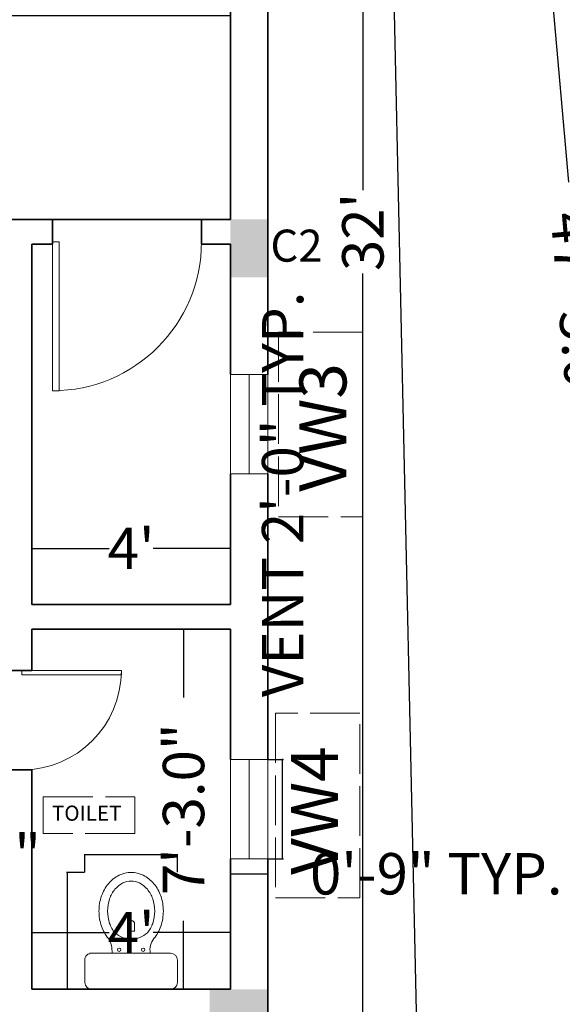
# Model space of a CAD drawing. Units: inches. Extents: x -269 to 4574, y -694 to 313.
# Tile 8 of 19: x 391 to 522, y -360 to -122. Entities that reach past the tile are written whole.
import ezdxf

# ---------------------------------------------------------------- set-up
doc = ezdxf.new("R2010")
doc.units = ezdxf.units.IN
doc.header["$MEASUREMENT"] = 0
doc.linetypes.add('ACAD_ISO02W100', pattern=[15, 12, -3])
for name, color, linetype, lineweight in [('A-ANNO-FRAM', 7, 'ACAD_ISO02W100', 13), ('A-ANNO-IDEN', 6, 'Continuous', 18), ('A-AREA-IDEN', 6, 'Continuous', 20), ('A-COLS', 5, 'Continuous', 35), ('A-COLS-IDEN', 6, 'Continuous', 18), ('A-FLOR-FIXT', 21, 'Continuous', 18), ('C-PROP', 7, 'Continuous', 25), ('DIMENSION', 5, 'Continuous', 18), ('DOORS', 3, 'Continuous', 18), ('WALL', 1, 'Continuous', 35), ('WINDOWS', 2, 'Continuous', 18)]:
    doc.layers.add(name, color=color, linetype=linetype, lineweight=lineweight)
doc.dimstyles.get("Standard").update_dxf_attribs({"dimtxt": 10, "dimasz": 0.18, "dimexe": 0.18, "dimexo": 0.0625, "dimgap": 0.09, "dimtad": 0, "dimdec": 1, "dimzin": 0, "dimdsep": 46, "dimlunit": 3, "dimtxsty": 'Standard', "dimcen": 0.09, "dimclrt": 7, "dimadec": 0, "dimazin": 0, "dimtfac": 1, "dimtdec": 1, "dimtofl": 0, "dimtmove": 0, "dimatfit": 3, "dimfxl": 1, "dimtolj": 1, "dimtzin": 0, "dimarcsym": 0})

# ---------------------------------------------------------------- blocks, each defined once
blk = doc.blocks.new('A$C00A665A6')
for p, q in [((0, 640), (0, 510)), ((40, 680), (500, 680)), ((540, 640), (540, 510)), ((40, 470), (500, 470)), ((158.6, 470), (158.6, 470)), ((250, 342.2), (290, 342.2)), ((250, 342.2), (250, 294.3)), ((251.5, 290.7), (259.5, 282.7)), ((280.5, 282.7), (288.5, 290.7)), ((290, 342.2), (290, 294.3)), ((259.5, 282.7), (280.5, 282.7))]:
    blk.add_line(p, q)
for points in [[(158.6, 470, -0.215497), (137.4, 384.1, 0.09084), (97.2, 312.9, 0.083285), (82.5, 225, 0.083285), (97.2, 137.1, 0.09084), (137.4, 65.9, 0.104065), (200, 16.4, 0.115836), (270, 0, 0.115836), (340, 16.4, 0.104065), (402.6, 65.9, 0.09084), (442.8, 137.1, 0.083285), (457.5, 225, 0.083285)], [(457.5, 225, 0.083285), (442.8, 312.9, 0.09084), (402.6, 384.1, -0.156524), (381.4, 470)], [(200, 433.6), (200, 433.6, 0.104065)], [(340, 433.6), (340, 433.6, 0.115836)], [(268.2, 388.7, 0.171753), (175.8, 352.1, 0.09084), (144.5, 296.5, 0.083285), (132.5, 225, 0.083285), (144.5, 153.5, 0.09084), (175.8, 97.9, 0.104065), (222.3, 61.2, 0.115836), (270, 50, 0.115836)], [(271.8, 388.7, -0.171753), (364.2, 352.1, -0.09084), (395.5, 296.5, -0.083285), (407.5, 225, -0.083285), (395.5, 153.5, -0.09084), (364.2, 97.9, -0.104065), (317.7, 61.2, -0.115836), (270, 50, -0.115836)]]:
    blk.add_lwpolyline(points, format="xyb")
for centre in [(200, 450), (340, 450)]:
    blk.add_circle(centre, 10)
for centre, radius, start, end in [((40, 640), 40, 90, 180), ((500, 640), 40, 0, 90), ((40, 510), 40, 180, 270), ((500, 510), 40, 270, 0), ((255, 294.3), 5, 180, 225), ((285, 294.3), 5, 315, 0)]:
    blk.add_arc(centre, radius, start, end)
blk = doc.blocks.new('*U3')
for p, q in [((0, 0), (0, -6)), ((40, 0), (40, -6))]:
    blk.add_line(p, q)
blk.add_lwpolyline([(0, 0), (0, 40), (1.75, 40), (1.75, 0)], close=True)
blk.add_arc((0, 0), 40, 0, 90)
blk = doc.blocks.new('*D20')
at = {"layer": 'Defpoints', "color": 0, "lineweight": 0, "transparency": 16777216}
for p in [(262.14, -122.44), (442.14, -121.56), (442.14, -122.44)]:
    blk.add_point(p, dxfattribs=at)
at = {"layer": 'DIMENSION', "color": 0, "lineweight": -2, "transparency": 16777216}
for p, q in [((262.14, -122.38), (262.14, -121.38)), ((262.32, -121.56), (343, -121.56)), ((441.96, -121.56), (361.27, -121.56)), ((442.14, -122.38), (442.14, -121.38))]:
    blk.add_line(p, q, dxfattribs=at)
at = {"layer": 'DIMENSION', "color": 0, "lineweight": 0, "transparency": 16777216}
for points in [[(262.32, -121.53), (262.32, -121.59), (262.14, -121.56)], [(441.96, -121.53), (441.96, -121.59), (442.14, -121.56)]]:
    blk.add_solid(points, dxfattribs=at)
at = {"layer": 'DIMENSION', "color": 0, "transparency": 16777216, "insert": (352.14, -121.56), "char_height": 10, "attachment_point": 5}
blk.add_mtext("\\A1;15'", dxfattribs=at)
blk = doc.blocks.new('*D23')
at = {"layer": 'Defpoints', "color": 0, "lineweight": 0, "transparency": 16777216}
for p in [(442.14, -250.22), (394.14, -263.73), (442.14, -263.73)]:
    blk.add_point(p, dxfattribs=at)
at = {"layer": 'DIMENSION', "color": 0, "lineweight": -2, "transparency": 16777216}
for p, q in [((394.14, -263.67), (394.14, -250.04)), ((394.32, -250.22), (412.81, -250.22)), ((441.96, -250.22), (423.47, -250.22)), ((442.14, -263.67), (442.14, -250.04))]:
    blk.add_line(p, q, dxfattribs=at)
at = {"layer": 'DIMENSION', "color": 0, "lineweight": 0, "transparency": 16777216}
for points in [[(394.32, -250.19), (394.32, -250.25), (394.14, -250.22)], [(441.96, -250.19), (441.96, -250.25), (442.14, -250.22)]]:
    blk.add_solid(points, dxfattribs=at)
at = {"layer": 'DIMENSION', "color": 0, "transparency": 16777216, "insert": (418.14, -250.22), "char_height": 10, "attachment_point": 5}
blk.add_mtext("\\A1;4'", dxfattribs=at)
blk = doc.blocks.new('*D24')
at = {"layer": 'Defpoints', "color": 0, "lineweight": 0, "transparency": 16777216}
for p in [(430.79, -269.73), (442.14, -269.73), (442.14, -356.73)]:
    blk.add_point(p, dxfattribs=at)
at = {"layer": 'DIMENSION', "color": 0, "lineweight": -2, "transparency": 16777216}
for p, q in [((442.07, -269.73), (430.61, -269.73)), ((430.79, -269.91), (430.79, -286.24)), ((430.79, -356.55), (430.79, -340.23)), ((442.07, -356.73), (430.61, -356.73))]:
    blk.add_line(p, q, dxfattribs=at)
at = {"layer": 'DIMENSION', "color": 0, "lineweight": 0, "transparency": 16777216}
for points in [[(430.76, -269.91), (430.82, -269.91), (430.79, -269.73)], [(430.76, -356.55), (430.82, -356.55), (430.79, -356.73)]]:
    blk.add_solid(points, dxfattribs=at)
at = {"layer": 'DIMENSION', "color": 0, "transparency": 16777216, "insert": (430.79, -313.23), "char_height": 10, "attachment_point": 5, "rotation": 90}
blk.add_mtext('\\A1;7\'-3.0"', dxfattribs=at)
blk = doc.blocks.new('*D27')
at = {"layer": 'Defpoints', "color": 0, "lineweight": 0, "transparency": 16777216}
for p in [(451.14, 18.27), (451.14, -365.73), (474.13, -365.73)]:
    blk.add_point(p, dxfattribs=at)
at = {"layer": 'DIMENSION', "color": 0, "lineweight": -2, "transparency": 16777216}
for p, q in [((451.2, 18.27), (474.31, 18.27)), ((474.13, 18.09), (474.13, -163.64)), ((474.13, -365.55), (474.13, -183.82)), ((451.2, -365.73), (474.31, -365.73))]:
    blk.add_line(p, q, dxfattribs=at)
at = {"layer": 'DIMENSION', "color": 0, "lineweight": 0, "transparency": 16777216}
for points in [[(474.1, 18.09), (474.16, 18.09), (474.13, 18.27)], [(474.1, -365.55), (474.16, -365.55), (474.13, -365.73)]]:
    blk.add_solid(points, dxfattribs=at)
at = {"layer": 'DIMENSION', "color": 0, "transparency": 16777216, "insert": (474.13, -173.73), "char_height": 10, "attachment_point": 5, "rotation": 90}
blk.add_mtext("\\A1;32'", dxfattribs=at)
blk = doc.blocks.new('*D35')
at = {"layer": 'Defpoints', "color": 0, "lineweight": 0, "transparency": 16777216}
for p in [(478.29, 88), (551.23, -476.8), (527.63, -478.86)]:
    blk.add_point(p, dxfattribs=at)
at = {"layer": 'DIMENSION', "color": 0, "lineweight": -2, "transparency": 16777216}
for p, q in [((478.36, 88.01), (502.07, 90.07)), ((501.91, 89.87), (523.81, -161.74)), ((551.21, -476.62), (529.31, -225.01)), ((527.69, -478.85), (551.41, -476.79))]:
    blk.add_line(p, q, dxfattribs=at)
at = {"layer": 'DIMENSION', "color": 0, "lineweight": 0, "transparency": 16777216}
for points in [[(501.94, 89.88), (501.88, 89.87), (501.89, 90.05)], [(551.24, -476.62), (551.18, -476.63), (551.23, -476.8)]]:
    blk.add_solid(points, dxfattribs=at)
at = {"layer": 'DIMENSION', "color": 0, "transparency": 16777216, "insert": (526.56, -193.38), "char_height": 10, "attachment_point": 5, "rotation": 274.9738}
blk.add_mtext('\\A1;47\'-5.0"', dxfattribs=at)
blk = doc.blocks.new('*D36')
at = {"layer": 'Defpoints', "color": 0, "lineweight": 0, "transparency": 16777216}
for p in [(442.14, -343.05), (394.14, -356.73), (442.14, -356.73)]:
    blk.add_point(p, dxfattribs=at)
at = {"layer": 'DIMENSION', "color": 0, "lineweight": -2, "transparency": 16777216}
for p, q in [((394.14, -356.67), (394.14, -342.87)), ((394.32, -343.05), (412.81, -343.05)), ((441.96, -343.05), (423.47, -343.05)), ((442.14, -356.67), (442.14, -342.87))]:
    blk.add_line(p, q, dxfattribs=at)
at = {"layer": 'DIMENSION', "color": 0, "lineweight": 0, "transparency": 16777216}
for points in [[(394.32, -343.02), (394.32, -343.08), (394.14, -343.05)], [(441.96, -343.02), (441.96, -343.08), (442.14, -343.05)]]:
    blk.add_solid(points, dxfattribs=at)
at = {"layer": 'DIMENSION', "color": 0, "transparency": 16777216, "insert": (418.14, -343.05), "char_height": 10, "attachment_point": 5}
blk.add_mtext("\\A1;4'", dxfattribs=at)
blk = doc.blocks.new('GLAZ-24IN')
blk.add_line((4.5, 24), (4.5, 0))
blk.add_lwpolyline([(0, 24), (9, 24), (9, 0), (0, 0)], close=True)
blk = doc.blocks.new('COLUMN-9x14-PLAN')
h = blk.add_hatch(color=256)
h.dxf.hatch_style = 1
h.paths.add_polyline_path([(9, 14), (0, 14), (0, 0), (9, 0), (9, 5)])
blk = doc.blocks.new('*D57')
at = {"layer": 'Defpoints', "color": 0, "lineweight": 0, "transparency": 16777216}
for p in [(406.93, -328.51), (402.7, -356.73), (406.93, -356.73)]:
    blk.add_point(p, dxfattribs=at)
at = {"layer": 'DIMENSION', "color": 0, "lineweight": -2, "transparency": 16777216}
for p, q in [((406.87, -328.51), (402.52, -328.51)), ((402.7, -328.69), (402.7, -356.55)), ((406.87, -356.73), (402.52, -356.73)), ((402.7, -356.73), (402.7, -356.91))]:
    blk.add_line(p, q, dxfattribs=at)
at = {"layer": 'DIMENSION', "color": 0, "lineweight": 0, "transparency": 16777216}
for points in [[(402.67, -328.69), (402.73, -328.69), (402.7, -328.51)], [(402.67, -356.55), (402.73, -356.55), (402.7, -356.73)]]:
    blk.add_solid(points, dxfattribs=at)
at = {"layer": 'DIMENSION', "color": 7, "transparency": 16777216, "insert": (402.7, -392), "char_height": 10, "attachment_point": 5, "rotation": 90}
blk.add_mtext('\\A1;WC 2\'-4"', dxfattribs=at)
blk = doc.blocks.new('*D58')
at = {"layer": 'Defpoints', "color": 0, "lineweight": 0, "transparency": 16777216}
for p in [(406.93, -324.28), (406.93, -328.51), (429.34, -328.51)]:
    blk.add_point(p, dxfattribs=at)
at = {"layer": 'DIMENSION', "color": 0, "lineweight": -2, "transparency": 16777216}
for p, q in [((406.93, -324.28), (406.75, -324.28)), ((406.93, -328.45), (406.93, -324.1)), ((429.16, -324.28), (407.11, -324.28)), ((429.34, -328.45), (429.34, -324.1))]:
    blk.add_line(p, q, dxfattribs=at)
at = {"layer": 'DIMENSION', "color": 0, "lineweight": 0, "transparency": 16777216}
for points in [[(407.11, -324.25), (407.11, -324.31), (406.93, -324.28)], [(429.16, -324.25), (429.16, -324.31), (429.34, -324.28)]]:
    blk.add_solid(points, dxfattribs=at)
at = {"layer": 'DIMENSION', "color": 7, "transparency": 16777216, "insert": (365.71, -324.28), "char_height": 10, "attachment_point": 5}
blk.add_mtext('\\A1;1\'-10 1/2"', dxfattribs=at)
blk = doc.blocks.new('*D59')
at = {"layer": 'Defpoints', "color": 0, "lineweight": 0, "transparency": 16777216}
for p in [(451.14, -301.23), (454.74, -301.23), (451.14, -325.23)]:
    blk.add_point(p, dxfattribs=at)
at = {"layer": 'DIMENSION', "color": 0, "lineweight": -2, "transparency": 16777216}
for p, q in [((451.2, -301.23), (454.92, -301.23)), ((454.74, -301.23), (454.74, -301.05)), ((454.74, -325.05), (454.74, -301.41)), ((451.2, -325.23), (454.92, -325.23))]:
    blk.add_line(p, q, dxfattribs=at)
at = {"layer": 'DIMENSION', "color": 0, "lineweight": 0, "transparency": 16777216}
for points in [[(454.71, -301.41), (454.77, -301.41), (454.74, -301.23)], [(454.71, -325.05), (454.77, -325.05), (454.74, -325.23)]]:
    blk.add_solid(points, dxfattribs=at)
at = {"layer": 'DIMENSION', "color": 7, "transparency": 16777216, "insert": (454.74, -237.15), "char_height": 10, "attachment_point": 5, "rotation": 90}
blk.add_mtext('\\A1;VENT 2\'-0" TYP.', dxfattribs=at)
blk = doc.blocks.new('*D60')
at = {"layer": 'Defpoints', "color": 0, "lineweight": 0, "transparency": 16777216}
for p in [(442.14, -325.23), (451.14, -325.23), (451.14, -328.83)]:
    blk.add_point(p, dxfattribs=at)
at = {"layer": 'DIMENSION', "color": 0, "lineweight": -2, "transparency": 16777216}
for p, q in [((442.14, -325.29), (442.14, -329.01)), ((451.14, -325.29), (451.14, -329.01)), ((442.32, -328.83), (450.96, -328.83)), ((451.14, -328.83), (451.32, -328.83))]:
    blk.add_line(p, q, dxfattribs=at)
at = {"layer": 'DIMENSION', "color": 0, "lineweight": 0, "transparency": 16777216}
for points in [[(442.32, -328.8), (442.32, -328.86), (442.14, -328.83)], [(450.96, -328.8), (450.96, -328.86), (451.14, -328.83)]]:
    blk.add_solid(points, dxfattribs=at)
at = {"layer": 'DIMENSION', "color": 7, "transparency": 16777216, "insert": (491.88, -328.83), "char_height": 10, "attachment_point": 5}
blk.add_mtext('\\A1;0\'-9" TYP.', dxfattribs=at)

msp = doc.modelspace()

# ---------------------------------------------------------------- linework, layer by layer
at = {"layer": 'A-ANNO-FRAM'}
for points in [[(474.13, -197.97), (453.77, -197.97), (453.77, -242.59), (474.13, -242.59)], [(473.41, -290.06), (453.05, -290.06), (453.05, -334.68), (473.41, -334.68)], [(396.91, -310.21), (419.03, -310.21), (419.03, -319.11), (396.91, -319.11)]]:
    msp.add_lwpolyline(points, close=True, dxfattribs=at)
at = {"layer": 'C-PROP'}
msp.add_line((490.29, -506.83), (478.29, 36.26), dxfattribs=at)
at = {"layer": 'WALL'}
for p, q in [((442.14, -100.23), (442.14, -170.73)), ((451.14, -100.23), (451.14, -208.23)), ((262.14, -170.73), (394.14, -170.73)), ((394.14, -170.73), (399.14, -170.73)), ((399.14, -170.73), (399.14, -176.73)), ((399.14, -170.73), (442.14, -170.73)), ((435.14, -170.73), (435.14, -176.73)), ((394.14, -176.73), (394.14, -263.73)), ((394.14, -176.73), (399.14, -176.73)), ((435.14, -176.73), (442.14, -176.73)), ((442.14, -176.73), (442.14, -208.23)), ((442.14, -232.23), (442.14, -263.73)), ((451.14, -232.23), (451.14, -301.23)), ((394.14, -263.73), (442.14, -263.73)), ((394.14, -269.73), (442.14, -269.73)), ((394.14, -269.73), (394.14, -279.73)), ((442.14, -269.73), (442.14, -301.23)), ((388.14, -279.73), (394.14, -279.73)), ((388.14, -303.73), (394.14, -303.73)), ((394.14, -303.73), (394.14, -356.73)), ((442.14, -325.23), (442.14, -356.73)), ((451.14, -325.23), (451.14, -365.73)), ((442.14, -356.73), (394.14, -356.73))]:
    msp.add_line(p, q, dxfattribs=at)

# ---------------------------------------------------------------- block references
at = {"layer": 'A-COLS'}
msp.add_blockref('COLUMN-9x14-PLAN', (442.12, -184.72), dxfattribs=at)
at = {"layer": 'A-COLS', "rotation": 90.0000000000004}
msp.add_blockref('COLUMN-9x14-PLAN', (451.14, -365.72), dxfattribs=at)
at = {"layer": 'A-FLOR-FIXT', "xscale": 0.0414981462726487, "yscale": 0.0414981462726487, "zscale": 0.0414981462726487, "rotation": 180}
msp.add_blockref('A$C00A665A6', (429.34, -328.51), dxfattribs=at)
at = {"layer": 'DOORS'}
for p, xscale, yscale, zscale, rotation in [((399.14, -176.13), -0.8996107347491925, 0.8996107347491925, 0.8996107347491925, 180), ((391.74, -279.73), 0.600602616892385, 0.600602616892385, 0.600602616892385, 270)]:
    msp.add_blockref('*U3', p, dxfattribs=dict(at, xscale=xscale, yscale=yscale, zscale=zscale, rotation=rotation))
at = {"layer": 'WINDOWS'}
for p in [(442.14, -232.23), (442.14, -325.23)]:
    msp.add_blockref('GLAZ-24IN', p, dxfattribs=at)

# ---------------------------------------------------------------- texts
at = {"layer": 'A-ANNO-IDEN'}
for s, p in [('VW3', (470.16, -236.52)), ('VW4', (468.1, -329.11))]:
    msp.add_text(s, height=11.343, rotation=90, dxfattribs=at).set_placement(p)
at = {"layer": 'A-AREA-IDEN'}
msp.add_text(' TOILET ', height=3.667, dxfattribs=at).set_placement((397.86, -316.02))
at = {"layer": 'A-COLS-IDEN'}
msp.add_text('C2', height=7.741, dxfattribs=at).set_placement((451.79, -180.93))

# ---------------------------------------------------------------- dimensions: what is measured, and where the dimension line sits
at = {"layer": 'DIMENSION'}
dim = msp.add_aligned_dim(p1=(478.29, 88), p2=(527.63, -478.86), distance=23.69, dimstyle='Standard', override={"dimclrd": 0, "dimclre": 0, "dimclrt": 0}, dxfattribs=at)
dim.commit()
dim.dimension.update_dxf_attribs({"geometry": '*D35', "text_midpoint": (526.56, -193.38)})
for base, p1, p2, angle, override, picture, middle in [((474.13, -365.73), (451.14, 18.27), (451.14, -365.73), 90, {"dimclrd": 0, "dimclre": 0, "dimclrt": 0}, '*D27', (474.13, -173.73)), ((430.79, -269.73), (442.14, -356.73), (442.14, -269.73), 90, {"dimclrd": 0, "dimclre": 0, "dimclrt": 0}, '*D24', (430.79, -313.23)), ((406.93, -324.28), (429.34, -328.51), (406.93, -328.51), 180, {"dimdec": 1, "dimlfac": 1, "dimrnd": 0, "dimzin": 1, "dimdsep": 46, "dimlunit": 4, "dimfrac": 2}, '*D58', (365.71, -324.28))]:
    dim = msp.add_linear_dim(base=base, p1=p1, p2=p2, angle=angle, dimstyle='Standard', override=override, dxfattribs=at)
    dim.commit()
    dim.dimension.update_dxf_attribs({"geometry": picture, "text_midpoint": middle})
for base, p1, p2, picture, middle in [((442.14, -121.56), (262.14, -122.44), (442.14, -122.44), '*D20', (352.14, -121.56)), ((442.14, -250.22), (394.14, -263.73), (442.14, -263.73), '*D23', (418.14, -250.22)), ((442.14, -343.05), (394.14, -356.73), (442.14, -356.73), '*D36', (418.14, -343.05))]:
    dim = msp.add_linear_dim(base=base, p1=p1, p2=p2, dimstyle='Standard', override={"dimclrd": 0, "dimclre": 0, "dimclrt": 0}, dxfattribs=at)
    dim.commit()
    dim.dimension.update_dxf_attribs({"geometry": picture, "text_midpoint": middle})
for base, p1, p2, angle, text, picture, middle in [((454.74, -301.23), (451.14, -325.23), (451.14, -301.23), 90, 'VENT <> TYP.', '*D59', (454.74, -237.15)), ((402.7, -356.73), (406.93, -328.51), (406.93, -356.73), 270, 'WC <>', '*D57', (402.7, -392))]:
    dim = msp.add_linear_dim(base=base, p1=p1, p2=p2, angle=angle, text=text, dimstyle='Standard', override={"dimdec": 1, "dimlfac": 1, "dimrnd": 0, "dimzin": 1, "dimdsep": 46, "dimlunit": 4, "dimfrac": 2}, dxfattribs=at)
    dim.commit()
    dim.dimension.update_dxf_attribs({"geometry": picture, "text_midpoint": middle})
dim = msp.add_linear_dim(base=(451.14, -328.83), p1=(442.14, -325.23), p2=(451.14, -325.23), text='<> TYP.', dimstyle='Standard', override={"dimdec": 1, "dimlfac": 1, "dimrnd": 0, "dimzin": 1, "dimdsep": 46, "dimlunit": 4, "dimfrac": 2}, dxfattribs=at)
dim.commit()
dim.dimension.update_dxf_attribs({"geometry": '*D60', "text_midpoint": (491.88, -328.83)})

doc.saveas('drawing.dxf')
